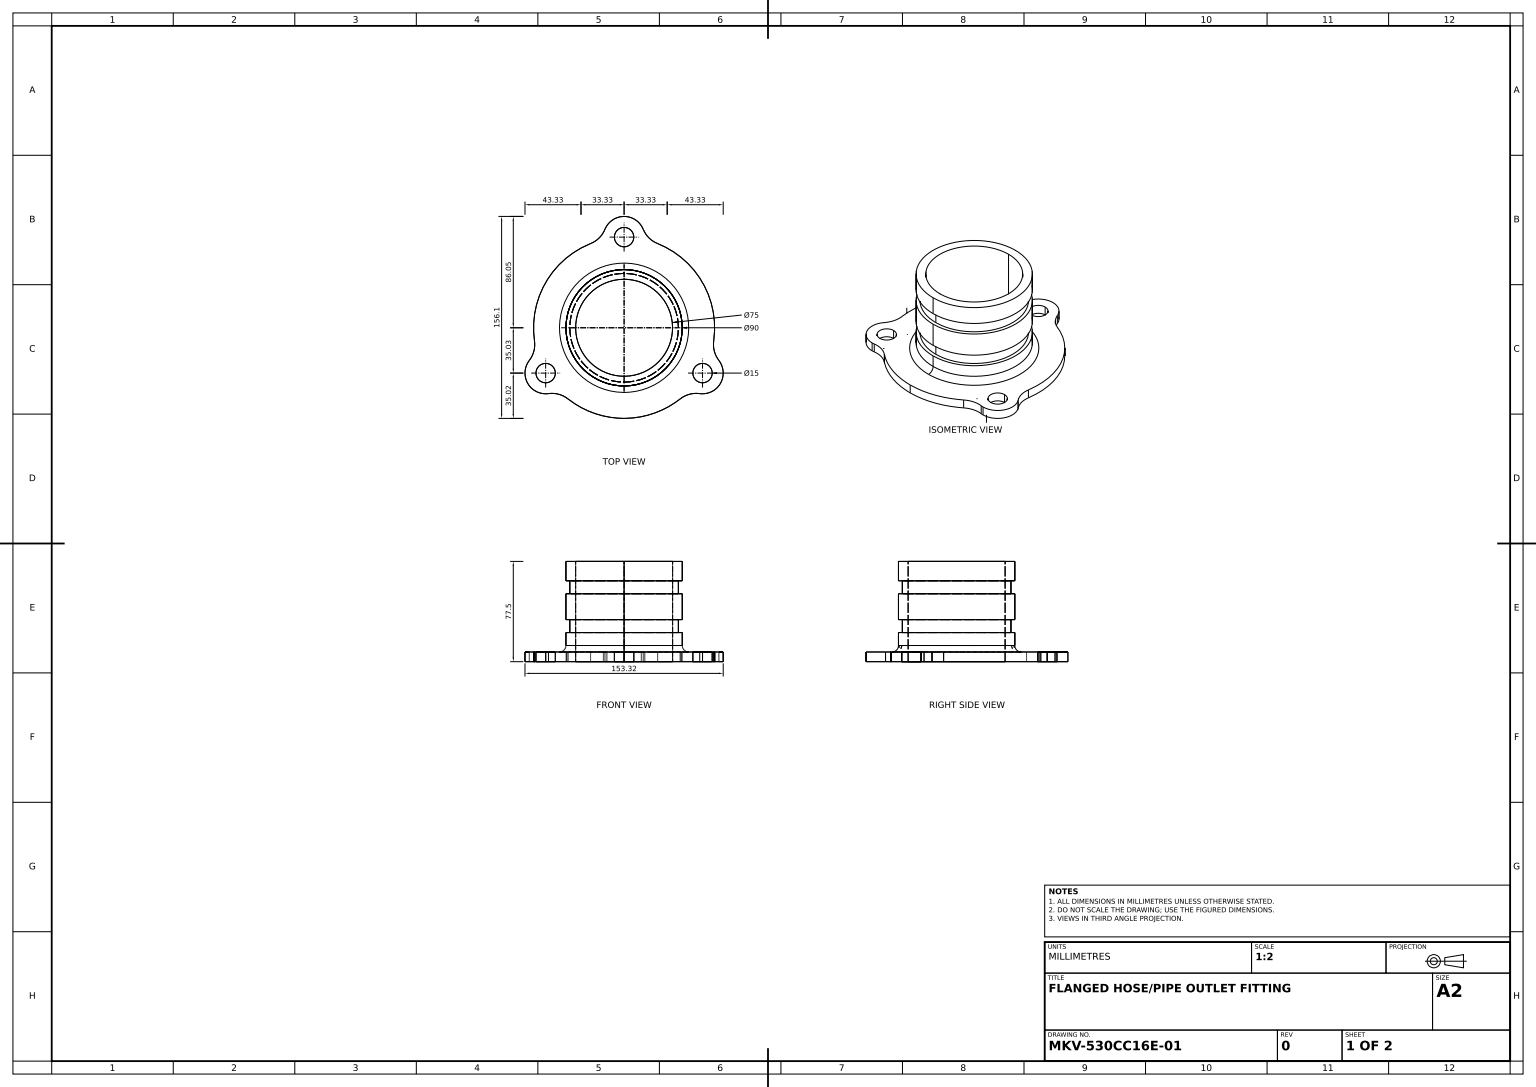
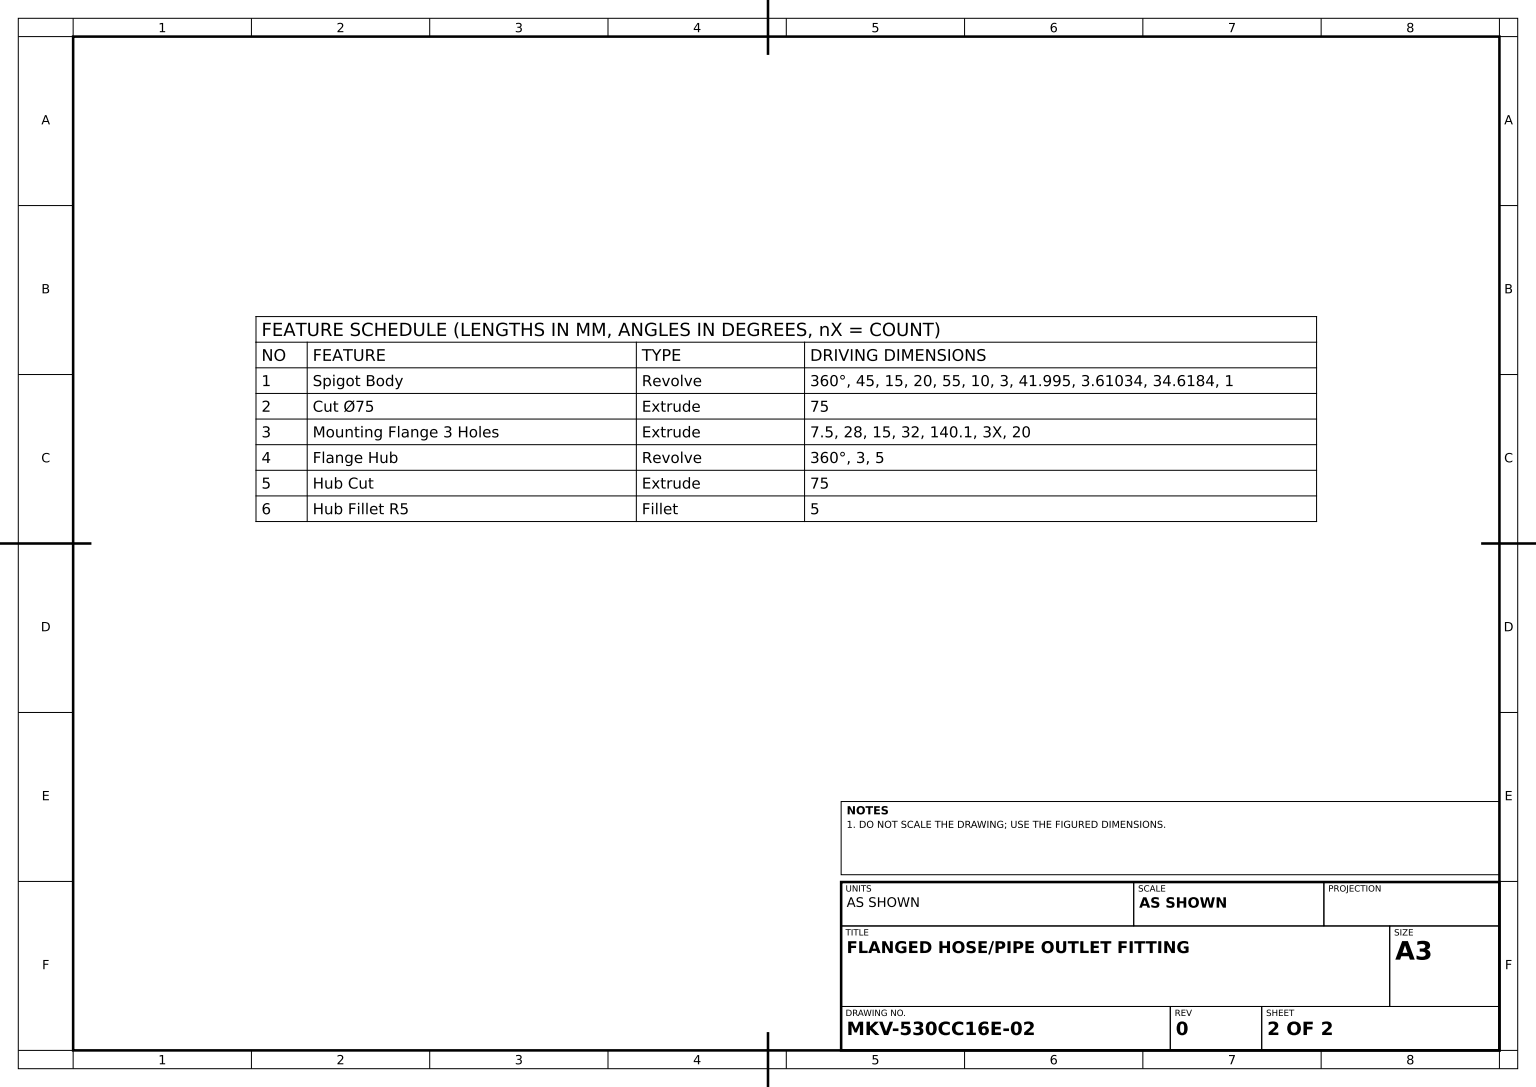
from build123d import *

# Parameters (mm, degrees)
CUT_CIRCLE_75_SKETCH_R        = 37.5
CUT_75_DEPTH                  = 85.113019206
MOUNTING_START                = -28
MOUNTING_FLANGE_SKETCH_R      = 7.5
MOUNTING_FLANGE_3_HOLES_DEPTH = 7.5
HUB_CUT_SKETCH_R              = 37.5
HUB_CUT_DEPTH                 = 139.879868922
HUB_FILLET_R5_R               = 5


with BuildPart() as part:
    # Spigot Profile Sketch → Spigot Body (revolve)
    with BuildSketch(Plane.XY, mode=Mode.PRIVATE) as spigot_body_sk:
        Polygon((0, -13.004960987), (0, 41.995039013), (-45, 41.995039013), (-45, 26.995039013), (-42, 26.995039013), (-42, 16.995039013), (-45, 16.995039013), (-45, -3.004960987), (-42, -3.004960987), (-42, -13.004960987), align=None)
    revolve(spigot_body_sk.sketch.rotate(Axis((0, 45.605381166, 0), (0, -1, 0)), 270), axis=Axis((0, 45.605381166, 0), (0, -1, 0)))

    # Cut Circle Ø75 Sketch → Cut Ø75 (cut, through all)
    with BuildSketch(Plane(origin=(0, 41.995039013, 0), x_dir=(1, 0, 0), z_dir=(0, 1, 0))):
        with Locations(Location((0, 0, 0), (0, 0, 270))):
            Circle(CUT_CIRCLE_75_SKETCH_R)
    extrude(amount=-CUT_75_DEPTH, mode=Mode.SUBTRACT)



with BuildPart() as body_2:
    # Mounting Flange Sketch → Mounting Flange 3 Holes (new body)
    with BuildSketch(Plane(origin=(0, 0, 0), x_dir=(1, 0, 0), z_dir=(0, 1, 0)).offset(MOUNTING_START)):
        with BuildLine():
            ThreePointArc((14.813512184, 76.09647474), (0, 86.05), (-14.813512184, 76.09647474))
            ThreePointArc((-14.813512184, 76.09647474), (-19.247651964, 69.453295695), (-25.927758901, 65.074986119))
            ThreePointArc((-25.927758901, 65.074986119), (-60.665079535, 35.025), (-69.32047058, -10.083395188))
            ThreePointArc((-69.32047058, -10.083395188), (-69.77214443, -18.057692283), (-73.308236355, -25.2193595))
            ThreePointArc((-73.308236355, -25.2193595), (-74.521485996, -43.025), (-58.494724172, -50.87711524))
            ThreePointArc((-58.494724172, -50.87711524), (-50.524492466, -51.395603412), (-43.392711679, -54.991590931))
            ThreePointArc((-43.392711679, -54.991590931), (0, -70.05), (43.392711679, -54.991590931))
            ThreePointArc((43.392711679, -54.991590931), (50.524492466, -51.395603412), (58.494724172, -50.87711524))
            ThreePointArc((58.494724172, -50.87711524), (74.521485996, -43.025), (73.308236355, -25.2193595))
            ThreePointArc((73.308236355, -25.2193595), (69.77214443, -18.057692283), (69.32047058, -10.083395188))
            ThreePointArc((69.32047058, -10.083395188), (60.665079535, 35.025), (25.927758901, 65.074986119))
            ThreePointArc((25.927758901, 65.074986119), (19.247651964, 69.453295695), (14.813512184, 76.09647474))
        make_face()
        with Locations(Location((0, 70.05, 0), (0, 0, 270))):
            Circle(MOUNTING_FLANGE_SKETCH_R, mode=Mode.SUBTRACT)
        with Locations(Location((60.665079535, -35.025, 0), (0, 0, 270))):
            Circle(MOUNTING_FLANGE_SKETCH_R, mode=Mode.SUBTRACT)
        with Locations(Location((-60.665079535, -35.025, 0), (0, 0, 270))):
            Circle(MOUNTING_FLANGE_SKETCH_R, mode=Mode.SUBTRACT)
    extrude(amount=-MOUNTING_FLANGE_3_HOLES_DEPTH)


with BuildPart() as part_1:
    add(part.part)

    add(body_2.part)  # Flange Hub merges body 2
    # Flange Hub Profile Sketch → Flange Hub (revolve)
    with BuildSketch(Plane.XY, mode=Mode.PRIVATE) as flange_hub_sk:
        Polygon((-45, -28), (0, -28), (0, -13.004960987), (-42, -13.004960987), (-45, -13.004960987), (-45, -23), align=None)
    revolve(flange_hub_sk.sketch.rotate(Axis((0, 0, 0), (0, -1, 0)), 270), axis=Axis((0, 0, 0), (0, -1, 0)))

    # Hub Cut Sketch → Hub Cut (cut, through all)
    with BuildSketch(Plane(origin=(0, 41.995039013, 0), x_dir=(1, 0, 0), z_dir=(0, 1, 0))):
        with Locations(Location((0, 0, 0), (0, 0, 270))):
            Circle(HUB_CUT_SKETCH_R)
    extrude(amount=-HUB_CUT_DEPTH, mode=Mode.SUBTRACT)

    # Hub Fillet R5
    hub_fillet_r5_edges = [part_1.edges().sort_by_distance(p)[0] for p in [
        (0, -28, -45),
    ]]
    fillet(hub_fillet_r5_edges, radius=HUB_FILLET_R5_R)


solid = part_1.part
